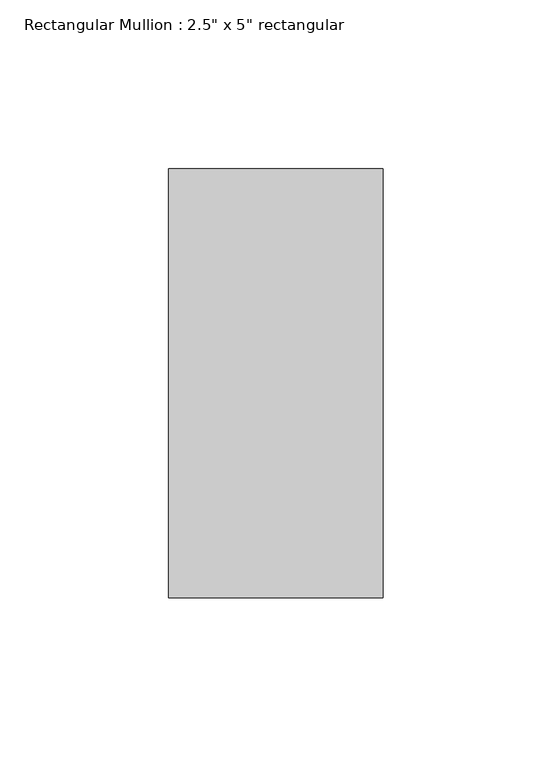
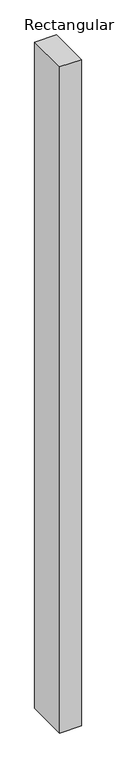
"""IFC4 building model written with IfcOpenShell, lengths in millimetres: member geometry."""

from ifc_helpers import new_model, si_unit, frame, origin, place, context, project, spatial, polyline, outline, extrude, source, transform, mapped, element, save


def member_820ab859(model_context):
    return source(origin(), model_context, "Body", "SweptSolid", [
        extrude(outline(polyline([(0.0, 63.5), (0.0, -63.5), (-63.5, -63.5), (-63.5, 63.5), (0.0, 63.5)])), frame((0.0, 0.0, -2065.7627175), z_axis=(0.0, 0.0, 1.0), x_axis=(1.0, 0.0, 0.0)), (0.0, 0.0, 1.0), 2065.7627175),
    ])


if __name__ == "__main__":
    model = new_model("IFC4")
    model_context = context("Model", 3, world=origin())
    ifc_project = project(units=[si_unit("LENGTHUNIT", "METRE", prefix="MILLI")], contexts=[model_context])
    site = spatial("IfcSite", under=ifc_project)
    building = spatial("IfcBuilding", under=site)
    placement = place(None, origin())
    member_shape = member_820ab859(model_context)
    element("IfcMember", 1, ObjectType="Rectangular Mullion : 2.5\" x 5\" rectangular", at=placement, inside=building, context=model_context, shape_type="MappedRepresentation", body=[
        mapped(member_shape, transform((0.0, 0.0, 0.0), x_axis=(1.0, 0.0, 0.0), y_axis=(0.0, 1.0, 0.0), z_axis=(0.0, 0.0, 1.0))),
    ])
    save(model, "model.ifc")

# Revit data of these elements
# Type "Rectangular Mullion : 2.5\" x 5\" rectangular"
#   built-in parameter 1007304 = 0.416667 (stored number, unit not read)
#   built-in parameter 1007301 = 0.104167 (stored number, unit not read)
#   built-in parameter 1007300 = 0.104167 (stored number, unit not read)
# Element 1 (IfcMember, "Rectangular Mullion : 2.5\" x 5\" rectangular")
#   Materials on its faces: "Iron, Ductile"
# Materials
#   "Iron, Ductile": class "Metal", colour RGB 0 0 0, transparency 0, Description = "Ductile cast iron", Cost = 0
